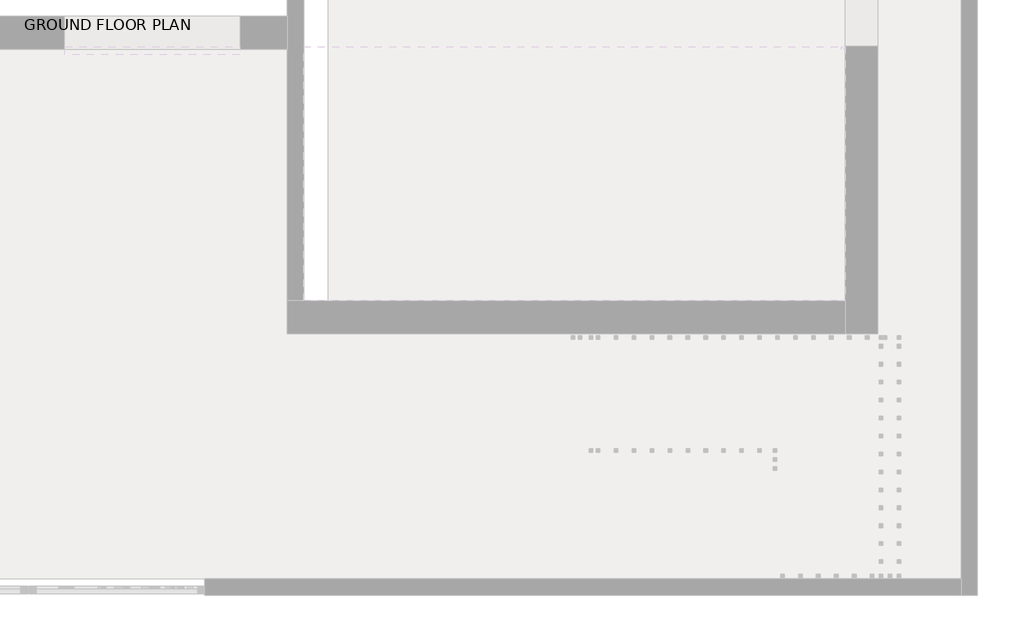
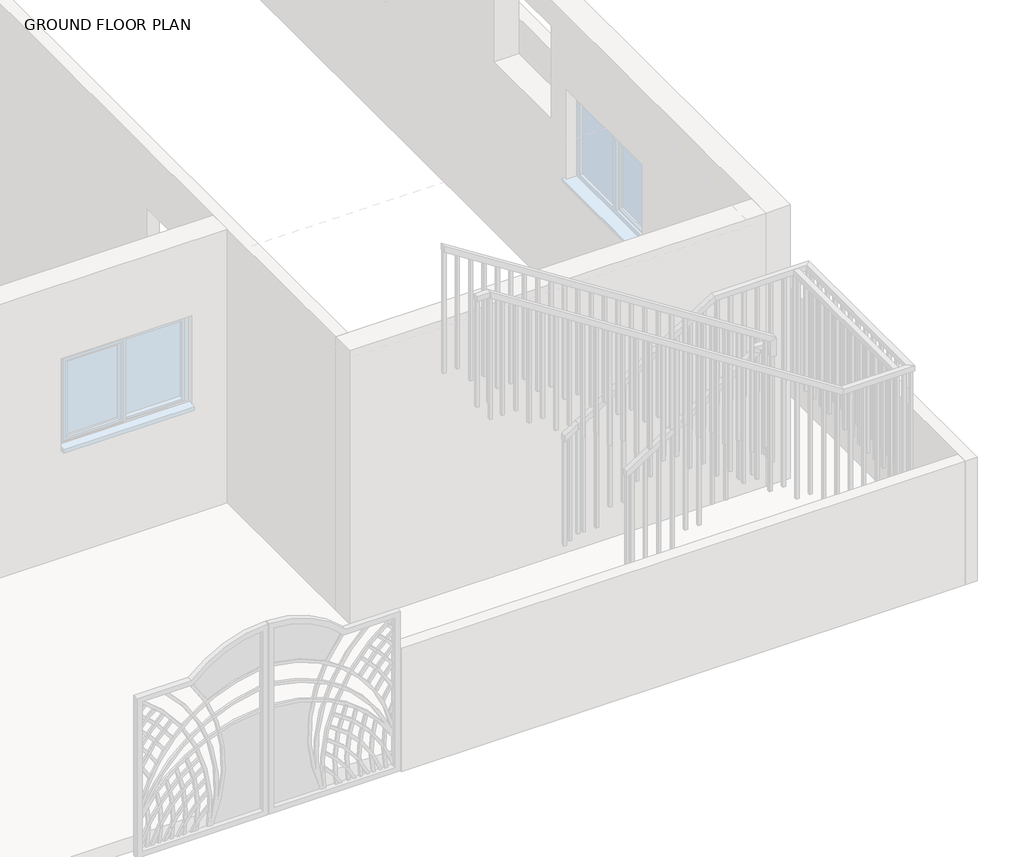
# One storey, part 15 of 23: 2 railings.
"""IFC4 building model written with IfcOpenShell, lengths in millimetres."""

from ifc_helpers import new_model, si_unit, frame, origin, place, context, project, spatial, polyline, outline, extrude, faceted_brep, element, save

model = new_model("IFC4")

# Units and contexts
model_context = context("Model", 3, world=origin())
ifc_project = project(units=[si_unit("LENGTHUNIT", "METRE", prefix="MILLI")], contexts=[model_context])

# Site, building, storey
site = spatial("IfcSite", under=ifc_project)
building = spatial("IfcBuilding", under=site)
storey = spatial("IfcBuildingStorey", under=building, Name="GROUND FLOOR PLAN", Elevation=487.68)

# Railings
placement = place(None, origin())
element("IfcRailing", 1, ObjectType="1100mm", at=placement, inside=storey, context=model_context, shape_type="SolidModel", body=[
    faceted_brep([(-8680.149573, -11007.9255223, 1912.8), (-8680.149573, -11007.9255223, 1853.4423995), (-8680.149573, -11057.9255223, 1853.4423995), (-8680.149573, -11057.9255223, 1912.8), (-7484.3306254, -11007.9255223, 2677.8717446), (-7434.3306254, -11007.9255223, 2650.5035914), (-7434.3306254, -11057.9255223, 2650.5035914), (-7484.3306254, -11057.9255223, 2677.8717446), (-7484.3306254, -11007.9255223, 2725.6), (-7434.3306254, -11007.9255223, 2675.6), (-7434.3306254, -11057.9255223, 2675.6), (-7484.3306254, -11057.9255223, 2725.6), (-7359.3306254, -11007.9255223, 2725.6), (-7359.3306254, -11007.9255223, 2675.6), (-7409.3306254, -11057.9255223, 2675.6), (-7409.3306254, -11057.9255223, 2725.6), (-7359.3306254, -11132.9255223, 2725.6), (-7359.3306254, -11132.9255223, 2675.6), (-7409.3306254, -11132.9255223, 2675.6), (-7409.3306254, -11132.9255223, 2725.6), (-7359.3306254, -11134.9255223, 2725.6), (-7409.3306254, -11134.9255223, 2725.6), (-7409.3306254, -11184.9255223, 2675.6), (-7359.3306254, -11184.9255223, 2675.6)], [[[0, 1, 2, 3]], [[1, 0, 4, 5]], [[2, 1, 5, 6]], [[3, 2, 6, 7]], [[0, 3, 7, 4]], [[5, 4, 8, 9]], [[6, 5, 9, 10]], [[7, 6, 10, 11]], [[4, 7, 11, 8]], [[9, 8, 12, 13]], [[10, 9, 13, 14]], [[11, 10, 14, 15]], [[8, 11, 15, 12]], [[13, 12, 16, 17]], [[14, 13, 17, 18]], [[15, 14, 18, 19]], [[12, 15, 19, 16]], [[20, 21, 22, 23]], [[17, 16, 20, 23]], [[18, 17, 23, 22]], [[19, 18, 22, 21]], [[16, 19, 21, 20]]]),
    faceted_brep([(-7359.3306254, -11134.9255223, 2725.6), (-7359.3306254, -11184.9255223, 2675.6), (-7409.3306254, -11184.9255223, 2675.6), (-7409.3306254, -11134.9255223, 2725.6), (-7359.3306254, -11134.9255223, 2855.9055527), (-7409.3306254, -11134.9255223, 2828.5415543), (-7409.3306254, -11184.9255223, 2828.5415543), (-7359.3306254, -11184.9255223, 2855.9055527)], [[[0, 1, 2, 3]], [[4, 5, 6, 7]], [[1, 0, 4, 7]], [[2, 1, 7, 6]], [[3, 2, 6, 5]], [[0, 3, 5, 4]]]),
    faceted_brep([(-7359.3306254, -11184.9255223, 2855.9055527), (-7409.3306254, -11184.9255223, 2828.5415543), (-7409.3306254, -11134.9255223, 2828.5415543), (-7359.3306254, -11134.9255223, 2855.9055527), (-10457.8773536, -11184.9255223, 4838.88), (-10457.8773536, -11134.9255223, 4838.88), (-10457.8773536, -11134.9255223, 4779.517542), (-10457.8773536, -11184.9255223, 4779.517542)], [[[0, 1, 2, 3]], [[4, 5, 6, 7]], [[1, 0, 4, 7]], [[2, 1, 7, 6]], [[3, 2, 6, 5]], [[0, 3, 5, 4]]]),
    extrude(outline(polyline([(3576.32, -10434.3306254), (4764.4483614, -10434.3306254), (4780.4475912, -10459.3306254), (3576.32, -10459.3306254), (3576.32, -10434.3306254)])), frame((0.0, -11172.4255223, 0.0), z_axis=(0.0, 1.0, 0.0), x_axis=(0.0, 0.0, 1.0)), (0.0, 0.0, 1.0), 25.0),
    extrude(outline(polyline([(3576.32, -10309.3306254), (4684.4522123, -10309.3306254), (4700.4514422, -10334.3306254), (3576.32, -10334.3306254), (3576.32, -10309.3306254)])), frame((0.0, -11172.4255223, 0.0), z_axis=(0.0, 1.0, 0.0), x_axis=(0.0, 0.0, 1.0)), (0.0, 0.0, 1.0), 25.0),
    extrude(outline(polyline([(3413.76, -10184.3306254), (4604.4560633, -10184.3306254), (4620.4552931, -10209.3306254), (3413.76, -10209.3306254), (3413.76, -10184.3306254)])), frame((0.0, -11172.4255223, 0.0), z_axis=(0.0, 1.0, 0.0), x_axis=(0.0, 0.0, 1.0)), (0.0, 0.0, 1.0), 25.0),
    extrude(outline(polyline([(3413.76, -10059.3306254), (4524.4599142, -10059.3306254), (4540.459144, -10084.3306254), (3413.76, -10084.3306254), (3413.76, -10059.3306254)])), frame((0.0, -11172.4255223, 0.0), z_axis=(0.0, 1.0, 0.0), x_axis=(0.0, 0.0, 1.0)), (0.0, 0.0, 1.0), 25.0),
    extrude(outline(polyline([(3251.2, -9934.3306254), (4444.4637652, -9934.3306254), (4460.462995, -9959.3306254), (3251.2, -9959.3306254), (3251.2, -9934.3306254)])), frame((0.0, -11172.4255223, 0.0), z_axis=(0.0, 1.0, 0.0), x_axis=(0.0, 0.0, 1.0)), (0.0, 0.0, 1.0), 25.0),
    extrude(outline(polyline([(3251.2, -9809.3306254), (4364.4676161, -9809.3306254), (4380.4668459, -9834.3306254), (3251.2, -9834.3306254), (3251.2, -9809.3306254)])), frame((0.0, -11172.4255223, 0.0), z_axis=(0.0, 1.0, 0.0), x_axis=(0.0, 0.0, 1.0)), (0.0, 0.0, 1.0), 25.0),
    extrude(outline(polyline([(3251.2, -9684.3306254), (4284.4714671, -9684.3306254), (4300.4706969, -9709.3306254), (3251.2, -9709.3306254), (3251.2, -9684.3306254)])), frame((0.0, -11172.4255223, 0.0), z_axis=(0.0, 1.0, 0.0), x_axis=(0.0, 0.0, 1.0)), (0.0, 0.0, 1.0), 25.0),
    extrude(outline(polyline([(3088.64, -9559.3306254), (4204.475318, -9559.3306254), (4220.4745478, -9584.3306254), (3088.64, -9584.3306254), (3088.64, -9559.3306254)])), frame((0.0, -11172.4255223, 0.0), z_axis=(0.0, 1.0, 0.0), x_axis=(0.0, 0.0, 1.0)), (0.0, 0.0, 1.0), 25.0),
    extrude(outline(polyline([(3088.64, -9434.3306254), (4124.479169, -9434.3306254), (4140.4783988, -9459.3306254), (3088.64, -9459.3306254), (3088.64, -9434.3306254)])), frame((0.0, -11172.4255223, 0.0), z_axis=(0.0, 1.0, 0.0), x_axis=(0.0, 0.0, 1.0)), (0.0, 0.0, 1.0), 25.0),
    extrude(outline(polyline([(2926.08, -9309.3306254), (4044.4830199, -9309.3306254), (4060.4822497, -9334.3306254), (2926.08, -9334.3306254), (2926.08, -9309.3306254)])), frame((0.0, -11172.4255223, 0.0), z_axis=(0.0, 1.0, 0.0), x_axis=(0.0, 0.0, 1.0)), (0.0, 0.0, 1.0), 25.0),
    extrude(outline(polyline([(2926.08, -9184.3306254), (3964.4868709, -9184.3306254), (3980.4861007, -9209.3306254), (2926.08, -9209.3306254), (2926.08, -9184.3306254)])), frame((0.0, -11172.4255223, 0.0), z_axis=(0.0, 1.0, 0.0), x_axis=(0.0, 0.0, 1.0)), (0.0, 0.0, 1.0), 25.0),
    extrude(outline(polyline([(2763.52, -9059.3306254), (3884.4907218, -9059.3306254), (3900.4899516, -9084.3306254), (2763.52, -9084.3306254), (2763.52, -9059.3306254)])), frame((0.0, -11172.4255223, 0.0), z_axis=(0.0, 1.0, 0.0), x_axis=(0.0, 0.0, 1.0)), (0.0, 0.0, 1.0), 25.0),
    extrude(outline(polyline([(2763.52, -8934.3306254), (3804.4945728, -8934.3306254), (3820.4938026, -8959.3306254), (2763.52, -8959.3306254), (2763.52, -8934.3306254)])), frame((0.0, -11172.4255223, 0.0), z_axis=(0.0, 1.0, 0.0), x_axis=(0.0, 0.0, 1.0)), (0.0, 0.0, 1.0), 25.0),
    extrude(outline(polyline([(2600.96, -8809.3306254), (3724.4984237, -8809.3306254), (3740.4976535, -8834.3306254), (2600.96, -8834.3306254), (2600.96, -8809.3306254)])), frame((0.0, -11172.4255223, 0.0), z_axis=(0.0, 1.0, 0.0), x_axis=(0.0, 0.0, 1.0)), (0.0, 0.0, 1.0), 25.0),
    extrude(outline(polyline([(2600.96, -8684.3306254), (3644.5022747, -8684.3306254), (3660.5015045, -8709.3306254), (2600.96, -8709.3306254), (2600.96, -8684.3306254)])), frame((0.0, -11172.4255223, 0.0), z_axis=(0.0, 1.0, 0.0), x_axis=(0.0, 0.0, 1.0)), (0.0, 0.0, 1.0), 25.0),
    extrude(outline(polyline([(2438.4, -8559.3306254), (3564.5061256, -8559.3306254), (3580.5053554, -8584.3306254), (2438.4, -8584.3306254), (2438.4, -8559.3306254)])), frame((0.0, -11172.4255223, 0.0), z_axis=(0.0, 1.0, 0.0), x_axis=(0.0, 0.0, 1.0)), (0.0, 0.0, 1.0), 25.0),
    extrude(outline(polyline([(2438.4, -8434.3306254), (3484.5099766, -8434.3306254), (3500.5092064, -8459.3306254), (2438.4, -8459.3306254), (2438.4, -8434.3306254)])), frame((0.0, -11172.4255223, 0.0), z_axis=(0.0, 1.0, 0.0), x_axis=(0.0, 0.0, 1.0)), (0.0, 0.0, 1.0), 25.0),
    extrude(outline(polyline([(2275.84, -8309.3306254), (3404.5138275, -8309.3306254), (3420.5130573, -8334.3306254), (2275.84, -8334.3306254), (2275.84, -8309.3306254)])), frame((0.0, -11172.4255223, 0.0), z_axis=(0.0, 1.0, 0.0), x_axis=(0.0, 0.0, 1.0)), (0.0, 0.0, 1.0), 25.0),
    extrude(outline(polyline([(2275.84, -8184.3306254), (3324.5176785, -8184.3306254), (3340.5169083, -8209.3306254), (2275.84, -8209.3306254), (2275.84, -8184.3306254)])), frame((0.0, -11172.4255223, 0.0), z_axis=(0.0, 1.0, 0.0), x_axis=(0.0, 0.0, 1.0)), (0.0, 0.0, 1.0), 25.0),
    extrude(outline(polyline([(2113.28, -8059.3306254), (3244.5215294, -8059.3306254), (3260.5207592, -8084.3306254), (2113.28, -8084.3306254), (2113.28, -8059.3306254)])), frame((0.0, -11172.4255223, 0.0), z_axis=(0.0, 1.0, 0.0), x_axis=(0.0, 0.0, 1.0)), (0.0, 0.0, 1.0), 25.0),
    extrude(outline(polyline([(2113.28, -7934.3306254), (3164.5253804, -7934.3306254), (3180.5246102, -7959.3306254), (2113.28, -7959.3306254), (2113.28, -7934.3306254)])), frame((0.0, -11172.4255223, 0.0), z_axis=(0.0, 1.0, 0.0), x_axis=(0.0, 0.0, 1.0)), (0.0, 0.0, 1.0), 25.0),
    extrude(outline(polyline([(1950.72, -7809.3306254), (3084.5292313, -7809.3306254), (3100.5284611, -7834.3306254), (1950.72, -7834.3306254), (1950.72, -7809.3306254)])), frame((0.0, -11172.4255223, 0.0), z_axis=(0.0, 1.0, 0.0), x_axis=(0.0, 0.0, 1.0)), (0.0, 0.0, 1.0), 25.0),
    extrude(outline(polyline([(1950.72, -7684.3306254), (3004.5330823, -7684.3306254), (3020.5323121, -7709.3306254), (1950.72, -7709.3306254), (1950.72, -7684.3306254)])), frame((0.0, -11172.4255223, 0.0), z_axis=(0.0, 1.0, 0.0), x_axis=(0.0, 0.0, 1.0)), (0.0, 0.0, 1.0), 25.0),
    extrude(outline(polyline([(1788.16, -7559.3306254), (2924.5369332, -7559.3306254), (2940.536163, -7584.3306254), (1788.16, -7584.3306254), (1788.16, -7559.3306254)])), frame((0.0, -11172.4255223, 0.0), z_axis=(0.0, 1.0, 0.0), x_axis=(0.0, 0.0, 1.0)), (0.0, 0.0, 1.0), 25.0),
    extrude(outline(polyline([(1788.16, -7434.3306254), (2844.5407841, -7434.3306254), (2860.540014, -7459.3306254), (1788.16, -7459.3306254), (1788.16, -7434.3306254)])), frame((0.0, -11172.4255223, 0.0), z_axis=(0.0, 1.0, 0.0), x_axis=(0.0, 0.0, 1.0)), (0.0, 0.0, 1.0), 25.0),
    extrude(outline(polyline([(-7396.8306254, -11082.9255223), (-7371.8306254, -11082.9255223), (-7371.8306254, -11107.9255223), (-7396.8306254, -11107.9255223), (-7396.8306254, -11082.9255223)])), frame((0.0, 0.0, 1625.6), z_axis=(0.0, 0.0, 1.0), x_axis=(1.0, 0.0, 0.0)), (0.0, 0.0, 1.0), 1050.0),
    extrude(outline(polyline([(2605.1944115, -7505.149573), (1463.04, -7505.149573), (1463.04, -7480.149573), (2621.1891352, -7480.149573), (2605.1944115, -7505.149573)])), frame((0.0, -11045.4255223, 0.0), z_axis=(0.0, 1.0, 0.0), x_axis=(0.0, 0.0, 1.0)), (0.0, 0.0, 1.0), 25.0),
    extrude(outline(polyline([(2525.2207932, -7630.149573), (1463.04, -7630.149573), (1463.04, -7605.149573), (2541.2155169, -7605.149573), (2525.2207932, -7630.149573)])), frame((0.0, -11045.4255223, 0.0), z_axis=(0.0, 1.0, 0.0), x_axis=(0.0, 0.0, 1.0)), (0.0, 0.0, 1.0), 25.0),
    extrude(outline(polyline([(2445.2471749, -7755.149573), (1300.48, -7755.149573), (1300.48, -7730.149573), (2461.2418986, -7730.149573), (2445.2471749, -7755.149573)])), frame((0.0, -11045.4255223, 0.0), z_axis=(0.0, 1.0, 0.0), x_axis=(0.0, 0.0, 1.0)), (0.0, 0.0, 1.0), 25.0),
    extrude(outline(polyline([(2365.2735566, -7880.149573), (1300.48, -7880.149573), (1300.48, -7855.149573), (2381.2682803, -7855.149573), (2365.2735566, -7880.149573)])), frame((0.0, -11045.4255223, 0.0), z_axis=(0.0, 1.0, 0.0), x_axis=(0.0, 0.0, 1.0)), (0.0, 0.0, 1.0), 25.0),
    extrude(outline(polyline([(2285.2999383, -8005.149573), (1137.92, -8005.149573), (1137.92, -7980.149573), (2301.294662, -7980.149573), (2285.2999383, -8005.149573)])), frame((0.0, -11045.4255223, 0.0), z_axis=(0.0, 1.0, 0.0), x_axis=(0.0, 0.0, 1.0)), (0.0, 0.0, 1.0), 25.0),
    extrude(outline(polyline([(2205.32632, -8130.149573), (1137.92, -8130.149573), (1137.92, -8105.149573), (2221.3210437, -8105.149573), (2205.32632, -8130.149573)])), frame((0.0, -11045.4255223, 0.0), z_axis=(0.0, 1.0, 0.0), x_axis=(0.0, 0.0, 1.0)), (0.0, 0.0, 1.0), 25.0),
    extrude(outline(polyline([(2125.3527017, -8255.149573), (975.36, -8255.149573), (975.36, -8230.149573), (2141.3474254, -8230.149573), (2125.3527017, -8255.149573)])), frame((0.0, -11045.4255223, 0.0), z_axis=(0.0, 1.0, 0.0), x_axis=(0.0, 0.0, 1.0)), (0.0, 0.0, 1.0), 25.0),
    extrude(outline(polyline([(2045.3790834, -8380.149573), (975.36, -8380.149573), (975.36, -8355.149573), (2061.3738071, -8355.149573), (2045.3790834, -8380.149573)])), frame((0.0, -11045.4255223, 0.0), z_axis=(0.0, 1.0, 0.0), x_axis=(0.0, 0.0, 1.0)), (0.0, 0.0, 1.0), 25.0),
    extrude(outline(polyline([(1965.4054651, -8505.149573), (812.8, -8505.149573), (812.8, -8480.149573), (1981.4001888, -8480.149573), (1965.4054651, -8505.149573)])), frame((0.0, -11045.4255223, 0.0), z_axis=(0.0, 1.0, 0.0), x_axis=(0.0, 0.0, 1.0)), (0.0, 0.0, 1.0), 25.0),
    extrude(outline(polyline([(1885.4318468, -8630.149573), (812.8, -8630.149573), (812.8, -8605.149573), (1901.4265705, -8605.149573), (1885.4318468, -8630.149573)])), frame((0.0, -11045.4255223, 0.0), z_axis=(0.0, 1.0, 0.0), x_axis=(0.0, 0.0, 1.0)), (0.0, 0.0, 1.0), 25.0),
    extrude(outline(polyline([(-7396.8306254, -11147.4255223), (-7371.8306254, -11147.4255223), (-7371.8306254, -11172.4255223), (-7396.8306254, -11172.4255223), (-7396.8306254, -11147.4255223)])), frame((0.0, 0.0, 1625.6), z_axis=(0.0, 0.0, 1.0), x_axis=(1.0, 0.0, 0.0)), (0.0, 0.0, 1.0), 1050.0),
    extrude(outline(polyline([(-7396.8306254, -11045.4255223), (-7396.8306254, -11020.4255223), (-7371.8306254, -11020.4255223), (-7371.8306254, -11045.4255223), (-7396.8306254, -11045.4255223)])), frame((0.0, 0.0, 1625.6), z_axis=(0.0, 0.0, 1.0), x_axis=(1.0, 0.0, 0.0)), (0.0, 0.0, 1.0), 1050.0),
    extrude(outline(polyline([(3576.32, -10432.8773536), (4763.5183122, -10432.8773536), (4779.517542, -10457.8773536), (3576.32, -10457.8773536), (3576.32, -10432.8773536)])), frame((0.0, -11172.4255223, 0.0), z_axis=(0.0, 1.0, 0.0), x_axis=(0.0, 0.0, 1.0)), (0.0, 0.0, 1.0), 25.0),
    extrude(outline(polyline([(1853.4423995, -8680.149573), (812.8, -8680.149573), (812.8, -8655.149573), (1869.4371231, -8655.149573), (1853.4423995, -8680.149573)])), frame((0.0, -11045.4255223, 0.0), z_axis=(0.0, 1.0, 0.0), x_axis=(0.0, 0.0, 1.0)), (0.0, 0.0, 1.0), 25.0),
])
element("IfcRailing", 2, ObjectType="1100mm", at=placement, inside=storey, context=model_context, shape_type="SolidModel", body=[
    faceted_brep([(-8680.149573, -10220.0521308, 1912.8), (-8680.149573, -10220.0521308, 1853.4423995), (-8680.149573, -10270.0521308, 1853.4423995), (-8680.149573, -10270.0521308, 1912.8), (-7409.7306254, -10220.0521308, 2725.6), (-7395.1045513, -10220.0521308, 2675.6), (-7395.1045513, -10270.0521308, 2675.6), (-7409.7306254, -10270.0521308, 2725.6), (-6495.8132565, -10220.0521308, 2725.6), (-6495.8132565, -10220.0521308, 2675.6), (-6545.8132565, -10270.0521308, 2675.6), (-6545.8132565, -10270.0521308, 2725.6), (-6495.8132565, -11933.6860066, 2725.6), (-6495.8132565, -11933.6860066, 2675.6), (-6545.8132565, -11883.6860066, 2675.6), (-6545.8132565, -11883.6860066, 2725.6), (-7155.718398, -11933.6860066, 2725.6), (-7170.3479429, -11933.6860066, 2675.6), (-7170.3479429, -11883.6860066, 2675.6), (-7155.718398, -11883.6860066, 2725.6), (-10457.8773536, -11933.6860066, 4838.88), (-10457.8773536, -11883.6860066, 4838.88), (-10457.8773536, -11883.6860066, 4779.517542), (-10457.8773536, -11933.6860066, 4779.517542)], [[[0, 1, 2, 3]], [[1, 0, 4, 5]], [[2, 1, 5, 6]], [[3, 2, 6, 7]], [[0, 3, 7, 4]], [[5, 4, 8, 9]], [[6, 5, 9, 10]], [[7, 6, 10, 11]], [[4, 7, 11, 8]], [[9, 8, 12, 13]], [[10, 9, 13, 14]], [[11, 10, 14, 15]], [[8, 11, 15, 12]], [[13, 12, 16, 17]], [[14, 13, 17, 18]], [[15, 14, 18, 19]], [[12, 15, 19, 16]], [[20, 21, 22, 23]], [[17, 16, 20, 23]], [[18, 17, 23, 22]], [[19, 18, 22, 21]], [[16, 19, 21, 20]]]),
    extrude(outline(polyline([(4691.8007425, -10320.8132565), (4707.7999723, -10345.8132565), (3576.32, -10345.8132565), (3576.32, -10320.8132565), (4691.8007425, -10320.8132565)])), frame((0.0, -11921.1860066, 0.0), z_axis=(0.0, 1.0, 0.0), x_axis=(0.0, 0.0, 1.0)), (0.0, 0.0, 1.0), 25.0),
    extrude(outline(polyline([(4611.8045935, -10195.8132565), (4627.8038233, -10220.8132565), (3576.32, -10220.8132565), (3576.32, -10195.8132565), (4611.8045935, -10195.8132565)])), frame((0.0, -11921.1860066, 0.0), z_axis=(0.0, 1.0, 0.0), x_axis=(0.0, 0.0, 1.0)), (0.0, 0.0, 1.0), 25.0),
    extrude(outline(polyline([(4531.8084444, -10070.8132565), (4547.8076742, -10095.8132565), (3413.76, -10095.8132565), (3413.76, -10070.8132565), (4531.8084444, -10070.8132565)])), frame((0.0, -11921.1860066, 0.0), z_axis=(0.0, 1.0, 0.0), x_axis=(0.0, 0.0, 1.0)), (0.0, 0.0, 1.0), 25.0),
    extrude(outline(polyline([(4451.8122954, -9945.8132565), (4467.8115252, -9970.8132565), (3413.76, -9970.8132565), (3413.76, -9945.8132565), (4451.8122954, -9945.8132565)])), frame((0.0, -11921.1860066, 0.0), z_axis=(0.0, 1.0, 0.0), x_axis=(0.0, 0.0, 1.0)), (0.0, 0.0, 1.0), 25.0),
    extrude(outline(polyline([(4371.8161463, -9820.8132565), (4387.8153761, -9845.8132565), (3251.2, -9845.8132565), (3251.2, -9820.8132565), (4371.8161463, -9820.8132565)])), frame((0.0, -11921.1860066, 0.0), z_axis=(0.0, 1.0, 0.0), x_axis=(0.0, 0.0, 1.0)), (0.0, 0.0, 1.0), 25.0),
    extrude(outline(polyline([(4291.8423995, -9695.8132565), (4307.8371231, -9720.8132565), (3251.2, -9720.8132565), (3251.2, -9695.8132565), (4291.8423995, -9695.8132565)])), frame((0.0, -11921.1860066, 0.0), z_axis=(0.0, 1.0, 0.0), x_axis=(0.0, 0.0, 1.0)), (0.0, 0.0, 1.0), 25.0),
    extrude(outline(polyline([(4211.8238482, -9570.8132565), (4227.823078, -9595.8132565), (3088.64, -9595.8132565), (3088.64, -9570.8132565), (4211.8238482, -9570.8132565)])), frame((0.0, -11921.1860066, 0.0), z_axis=(0.0, 1.0, 0.0), x_axis=(0.0, 0.0, 1.0)), (0.0, 0.0, 1.0), 25.0),
    extrude(outline(polyline([(4131.8276992, -9445.8132565), (4147.826929, -9470.8132565), (3088.64, -9470.8132565), (3088.64, -9445.8132565), (4131.8276992, -9445.8132565)])), frame((0.0, -11921.1860066, 0.0), z_axis=(0.0, 1.0, 0.0), x_axis=(0.0, 0.0, 1.0)), (0.0, 0.0, 1.0), 25.0),
    extrude(outline(polyline([(4051.8315501, -9320.8132565), (4067.8307799, -9345.8132565), (2926.08, -9345.8132565), (2926.08, -9320.8132565), (4051.8315501, -9320.8132565)])), frame((0.0, -11921.1860066, 0.0), z_axis=(0.0, 1.0, 0.0), x_axis=(0.0, 0.0, 1.0)), (0.0, 0.0, 1.0), 25.0),
    extrude(outline(polyline([(3971.835401, -9195.8132565), (3987.8346309, -9220.8132565), (2926.08, -9220.8132565), (2926.08, -9195.8132565), (3971.835401, -9195.8132565)])), frame((0.0, -11921.1860066, 0.0), z_axis=(0.0, 1.0, 0.0), x_axis=(0.0, 0.0, 1.0)), (0.0, 0.0, 1.0), 25.0),
    extrude(outline(polyline([(3891.839252, -9070.8132565), (3907.8384818, -9095.8132565), (2763.52, -9095.8132565), (2763.52, -9070.8132565), (3891.839252, -9070.8132565)])), frame((0.0, -11921.1860066, 0.0), z_axis=(0.0, 1.0, 0.0), x_axis=(0.0, 0.0, 1.0)), (0.0, 0.0, 1.0), 25.0),
    extrude(outline(polyline([(3811.8431029, -8945.8132565), (3827.8423328, -8970.8132565), (2763.52, -8970.8132565), (2763.52, -8945.8132565), (3811.8431029, -8945.8132565)])), frame((0.0, -11921.1860066, 0.0), z_axis=(0.0, 1.0, 0.0), x_axis=(0.0, 0.0, 1.0)), (0.0, 0.0, 1.0), 25.0),
    extrude(outline(polyline([(3731.8469539, -8820.8132565), (3747.8461837, -8845.8132565), (2600.96, -8845.8132565), (2600.96, -8820.8132565), (3731.8469539, -8820.8132565)])), frame((0.0, -11921.1860066, 0.0), z_axis=(0.0, 1.0, 0.0), x_axis=(0.0, 0.0, 1.0)), (0.0, 0.0, 1.0), 25.0),
    extrude(outline(polyline([(3651.8508048, -8695.8132565), (3667.8500347, -8720.8132565), (2600.96, -8720.8132565), (2600.96, -8695.8132565), (3651.8508048, -8695.8132565)])), frame((0.0, -11921.1860066, 0.0), z_axis=(0.0, 1.0, 0.0), x_axis=(0.0, 0.0, 1.0)), (0.0, 0.0, 1.0), 25.0),
    extrude(outline(polyline([(3571.8546558, -8570.8132565), (3587.8538856, -8595.8132565), (2438.4, -8595.8132565), (2438.4, -8570.8132565), (3571.8546558, -8570.8132565)])), frame((0.0, -11921.1860066, 0.0), z_axis=(0.0, 1.0, 0.0), x_axis=(0.0, 0.0, 1.0)), (0.0, 0.0, 1.0), 25.0),
    extrude(outline(polyline([(3491.8585067, -8445.8132565), (3507.8577365, -8470.8132565), (2438.4, -8470.8132565), (2438.4, -8445.8132565), (3491.8585067, -8445.8132565)])), frame((0.0, -11921.1860066, 0.0), z_axis=(0.0, 1.0, 0.0), x_axis=(0.0, 0.0, 1.0)), (0.0, 0.0, 1.0), 25.0),
    extrude(outline(polyline([(3411.8623577, -8320.8132565), (3427.8615875, -8345.8132565), (2275.84, -8345.8132565), (2275.84, -8320.8132565), (3411.8623577, -8320.8132565)])), frame((0.0, -11921.1860066, 0.0), z_axis=(0.0, 1.0, 0.0), x_axis=(0.0, 0.0, 1.0)), (0.0, 0.0, 1.0), 25.0),
    extrude(outline(polyline([(3331.8662086, -8195.8132565), (3347.8654384, -8220.8132565), (2275.84, -8220.8132565), (2275.84, -8195.8132565), (3331.8662086, -8195.8132565)])), frame((0.0, -11921.1860066, 0.0), z_axis=(0.0, 1.0, 0.0), x_axis=(0.0, 0.0, 1.0)), (0.0, 0.0, 1.0), 25.0),
    extrude(outline(polyline([(3251.8700596, -8070.8132565), (3267.8692894, -8095.8132565), (2113.28, -8095.8132565), (2113.28, -8070.8132565), (3251.8700596, -8070.8132565)])), frame((0.0, -11921.1860066, 0.0), z_axis=(0.0, 1.0, 0.0), x_axis=(0.0, 0.0, 1.0)), (0.0, 0.0, 1.0), 25.0),
    extrude(outline(polyline([(3171.8739105, -7945.8132565), (3187.8731403, -7970.8132565), (2113.28, -7970.8132565), (2113.28, -7945.8132565), (3171.8739105, -7945.8132565)])), frame((0.0, -11921.1860066, 0.0), z_axis=(0.0, 1.0, 0.0), x_axis=(0.0, 0.0, 1.0)), (0.0, 0.0, 1.0), 25.0),
    extrude(outline(polyline([(3091.8777615, -7820.8132565), (3107.8769913, -7845.8132565), (1950.72, -7845.8132565), (1950.72, -7820.8132565), (3091.8777615, -7820.8132565)])), frame((0.0, -11921.1860066, 0.0), z_axis=(0.0, 1.0, 0.0), x_axis=(0.0, 0.0, 1.0)), (0.0, 0.0, 1.0), 25.0),
    extrude(outline(polyline([(3011.8816124, -7695.8132565), (3027.8808422, -7720.8132565), (1950.72, -7720.8132565), (1950.72, -7695.8132565), (3011.8816124, -7695.8132565)])), frame((0.0, -11921.1860066, 0.0), z_axis=(0.0, 1.0, 0.0), x_axis=(0.0, 0.0, 1.0)), (0.0, 0.0, 1.0), 25.0),
    extrude(outline(polyline([(2931.8854634, -7570.8132565), (2947.8846932, -7595.8132565), (1788.16, -7595.8132565), (1788.16, -7570.8132565), (2931.8854634, -7570.8132565)])), frame((0.0, -11921.1860066, 0.0), z_axis=(0.0, 1.0, 0.0), x_axis=(0.0, 0.0, 1.0)), (0.0, 0.0, 1.0), 25.0),
    extrude(outline(polyline([(2851.8893143, -7445.8132565), (2867.8885441, -7470.8132565), (1788.16, -7470.8132565), (1788.16, -7445.8132565), (2851.8893143, -7445.8132565)])), frame((0.0, -11921.1860066, 0.0), z_axis=(0.0, 1.0, 0.0), x_axis=(0.0, 0.0, 1.0)), (0.0, 0.0, 1.0), 25.0),
    extrude(outline(polyline([(2771.8931653, -7320.8132565), (2787.8923951, -7345.8132565), (1625.6, -7345.8132565), (1625.6, -7320.8132565), (2771.8931653, -7320.8132565)])), frame((0.0, -11921.1860066, 0.0), z_axis=(0.0, 1.0, 0.0), x_axis=(0.0, 0.0, 1.0)), (0.0, 0.0, 1.0), 25.0),
    extrude(outline(polyline([(2691.8970162, -7195.8132565), (2707.896246, -7220.8132565), (1625.6, -7220.8132565), (1625.6, -7195.8132565), (2691.8970162, -7195.8132565)])), frame((0.0, -11921.1860066, 0.0), z_axis=(0.0, 1.0, 0.0), x_axis=(0.0, 0.0, 1.0)), (0.0, 0.0, 1.0), 25.0),
    extrude(outline(polyline([(-7070.8132565, -11921.1860066), (-7095.8132565, -11921.1860066), (-7095.8132565, -11896.1860066), (-7070.8132565, -11896.1860066), (-7070.8132565, -11921.1860066)])), frame((0.0, 0.0, 1625.6), z_axis=(0.0, 0.0, 1.0), x_axis=(1.0, 0.0, 0.0)), (0.0, 0.0, 1.0), 1050.0),
    extrude(outline(polyline([(-6945.8132565, -11921.1860066), (-6970.8132565, -11921.1860066), (-6970.8132565, -11896.1860066), (-6945.8132565, -11896.1860066), (-6945.8132565, -11921.1860066)])), frame((0.0, 0.0, 1625.6), z_axis=(0.0, 0.0, 1.0), x_axis=(1.0, 0.0, 0.0)), (0.0, 0.0, 1.0), 1050.0),
    extrude(outline(polyline([(-6820.8132565, -11921.1860066), (-6845.8132565, -11921.1860066), (-6845.8132565, -11896.1860066), (-6820.8132565, -11896.1860066), (-6820.8132565, -11921.1860066)])), frame((0.0, 0.0, 1625.6), z_axis=(0.0, 0.0, 1.0), x_axis=(1.0, 0.0, 0.0)), (0.0, 0.0, 1.0), 1050.0),
    extrude(outline(polyline([(-6695.8132565, -11921.1860066), (-6720.8132565, -11921.1860066), (-6720.8132565, -11896.1860066), (-6695.8132565, -11896.1860066), (-6695.8132565, -11921.1860066)])), frame((0.0, 0.0, 1625.6), z_axis=(0.0, 0.0, 1.0), x_axis=(1.0, 0.0, 0.0)), (0.0, 0.0, 1.0), 1050.0),
    extrude(outline(polyline([(-6570.8132565, -11921.1860066), (-6595.8132565, -11921.1860066), (-6595.8132565, -11896.1860066), (-6570.8132565, -11896.1860066), (-6570.8132565, -11921.1860066)])), frame((0.0, 0.0, 1625.6), z_axis=(0.0, 0.0, 1.0), x_axis=(1.0, 0.0, 0.0)), (0.0, 0.0, 1.0), 1050.0),
    extrude(outline(polyline([(-6508.3132565, -11795.0521308), (-6508.3132565, -11820.0521308), (-6533.3132565, -11820.0521308), (-6533.3132565, -11795.0521308), (-6508.3132565, -11795.0521308)])), frame((0.0, 0.0, 1625.6), z_axis=(0.0, 0.0, 1.0), x_axis=(1.0, 0.0, 0.0)), (0.0, 0.0, 1.0), 1050.0),
    extrude(outline(polyline([(-6508.3132565, -11670.0521308), (-6508.3132565, -11695.0521308), (-6533.3132565, -11695.0521308), (-6533.3132565, -11670.0521308), (-6508.3132565, -11670.0521308)])), frame((0.0, 0.0, 1625.6), z_axis=(0.0, 0.0, 1.0), x_axis=(1.0, 0.0, 0.0)), (0.0, 0.0, 1.0), 1050.0),
    extrude(outline(polyline([(-6508.3132565, -11545.0521308), (-6508.3132565, -11570.0521308), (-6533.3132565, -11570.0521308), (-6533.3132565, -11545.0521308), (-6508.3132565, -11545.0521308)])), frame((0.0, 0.0, 1625.6), z_axis=(0.0, 0.0, 1.0), x_axis=(1.0, 0.0, 0.0)), (0.0, 0.0, 1.0), 1050.0),
    extrude(outline(polyline([(-6508.3132565, -11420.0521308), (-6508.3132565, -11445.0521308), (-6533.3132565, -11445.0521308), (-6533.3132565, -11420.0521308), (-6508.3132565, -11420.0521308)])), frame((0.0, 0.0, 1625.6), z_axis=(0.0, 0.0, 1.0), x_axis=(1.0, 0.0, 0.0)), (0.0, 0.0, 1.0), 1050.0),
    extrude(outline(polyline([(-6508.3132565, -11295.0521308), (-6508.3132565, -11320.0521308), (-6533.3132565, -11320.0521308), (-6533.3132565, -11295.0521308), (-6508.3132565, -11295.0521308)])), frame((0.0, 0.0, 1625.6), z_axis=(0.0, 0.0, 1.0), x_axis=(1.0, 0.0, 0.0)), (0.0, 0.0, 1.0), 1050.0),
    extrude(outline(polyline([(-6508.3132565, -11170.0521308), (-6508.3132565, -11195.0521308), (-6533.3132565, -11195.0521308), (-6533.3132565, -11170.0521308), (-6508.3132565, -11170.0521308)])), frame((0.0, 0.0, 1625.6), z_axis=(0.0, 0.0, 1.0), x_axis=(1.0, 0.0, 0.0)), (0.0, 0.0, 1.0), 1050.0),
    extrude(outline(polyline([(-6508.3132565, -11045.0521308), (-6508.3132565, -11070.0521308), (-6533.3132565, -11070.0521308), (-6533.3132565, -11045.0521308), (-6508.3132565, -11045.0521308)])), frame((0.0, 0.0, 1625.6), z_axis=(0.0, 0.0, 1.0), x_axis=(1.0, 0.0, 0.0)), (0.0, 0.0, 1.0), 1050.0),
    extrude(outline(polyline([(-6508.3132565, -10920.0521308), (-6508.3132565, -10945.0521308), (-6533.3132565, -10945.0521308), (-6533.3132565, -10920.0521308), (-6508.3132565, -10920.0521308)])), frame((0.0, 0.0, 1625.6), z_axis=(0.0, 0.0, 1.0), x_axis=(1.0, 0.0, 0.0)), (0.0, 0.0, 1.0), 1050.0),
    extrude(outline(polyline([(-6508.3132565, -10795.0521308), (-6508.3132565, -10820.0521308), (-6533.3132565, -10820.0521308), (-6533.3132565, -10795.0521308), (-6508.3132565, -10795.0521308)])), frame((0.0, 0.0, 1625.6), z_axis=(0.0, 0.0, 1.0), x_axis=(1.0, 0.0, 0.0)), (0.0, 0.0, 1.0), 1050.0),
    extrude(outline(polyline([(-6508.3132565, -10670.0521308), (-6508.3132565, -10695.0521308), (-6533.3132565, -10695.0521308), (-6533.3132565, -10670.0521308), (-6508.3132565, -10670.0521308)])), frame((0.0, 0.0, 1625.6), z_axis=(0.0, 0.0, 1.0), x_axis=(1.0, 0.0, 0.0)), (0.0, 0.0, 1.0), 1050.0),
    extrude(outline(polyline([(-6508.3132565, -10545.0521308), (-6508.3132565, -10570.0521308), (-6533.3132565, -10570.0521308), (-6533.3132565, -10545.0521308), (-6508.3132565, -10545.0521308)])), frame((0.0, 0.0, 1625.6), z_axis=(0.0, 0.0, 1.0), x_axis=(1.0, 0.0, 0.0)), (0.0, 0.0, 1.0), 1050.0),
    extrude(outline(polyline([(-6508.3132565, -10420.0521308), (-6508.3132565, -10445.0521308), (-6533.3132565, -10445.0521308), (-6533.3132565, -10420.0521308), (-6508.3132565, -10420.0521308)])), frame((0.0, 0.0, 1625.6), z_axis=(0.0, 0.0, 1.0), x_axis=(1.0, 0.0, 0.0)), (0.0, 0.0, 1.0), 1050.0),
    extrude(outline(polyline([(-6508.3132565, -10295.0521308), (-6508.3132565, -10320.0521308), (-6533.3132565, -10320.0521308), (-6533.3132565, -10295.0521308), (-6508.3132565, -10295.0521308)])), frame((0.0, 0.0, 1625.6), z_axis=(0.0, 0.0, 1.0), x_axis=(1.0, 0.0, 0.0)), (0.0, 0.0, 1.0), 1050.0),
    extrude(outline(polyline([(-6630.149573, -10232.5521308), (-6605.149573, -10232.5521308), (-6605.149573, -10257.5521308), (-6630.149573, -10257.5521308), (-6630.149573, -10232.5521308)])), frame((0.0, 0.0, 1625.6), z_axis=(0.0, 0.0, 1.0), x_axis=(1.0, 0.0, 0.0)), (0.0, 0.0, 1.0), 1050.0),
    extrude(outline(polyline([(-6755.149573, -10232.5521308), (-6730.149573, -10232.5521308), (-6730.149573, -10257.5521308), (-6755.149573, -10257.5521308), (-6755.149573, -10232.5521308)])), frame((0.0, 0.0, 1625.6), z_axis=(0.0, 0.0, 1.0), x_axis=(1.0, 0.0, 0.0)), (0.0, 0.0, 1.0), 1050.0),
    extrude(outline(polyline([(-6880.149573, -10232.5521308), (-6855.149573, -10232.5521308), (-6855.149573, -10257.5521308), (-6880.149573, -10257.5521308), (-6880.149573, -10232.5521308)])), frame((0.0, 0.0, 1625.6), z_axis=(0.0, 0.0, 1.0), x_axis=(1.0, 0.0, 0.0)), (0.0, 0.0, 1.0), 1050.0),
    extrude(outline(polyline([(-7005.149573, -10232.5521308), (-6980.149573, -10232.5521308), (-6980.149573, -10257.5521308), (-7005.149573, -10257.5521308), (-7005.149573, -10232.5521308)])), frame((0.0, 0.0, 1625.6), z_axis=(0.0, 0.0, 1.0), x_axis=(1.0, 0.0, 0.0)), (0.0, 0.0, 1.0), 1050.0),
    extrude(outline(polyline([(-7130.149573, -10232.5521308), (-7105.149573, -10232.5521308), (-7105.149573, -10257.5521308), (-7130.149573, -10257.5521308), (-7130.149573, -10232.5521308)])), frame((0.0, 0.0, 1625.6), z_axis=(0.0, 0.0, 1.0), x_axis=(1.0, 0.0, 0.0)), (0.0, 0.0, 1.0), 1050.0),
    extrude(outline(polyline([(-7255.149573, -10232.5521308), (-7230.149573, -10232.5521308), (-7230.149573, -10257.5521308), (-7255.149573, -10257.5521308), (-7255.149573, -10232.5521308)])), frame((0.0, 0.0, 1625.6), z_axis=(0.0, 0.0, 1.0), x_axis=(1.0, 0.0, 0.0)), (0.0, 0.0, 1.0), 1050.0),
    extrude(outline(polyline([(-7380.149573, -10232.5521308), (-7355.149573, -10232.5521308), (-7355.149573, -10257.5521308), (-7380.149573, -10257.5521308), (-7380.149573, -10232.5521308)])), frame((0.0, 0.0, 1625.6), z_axis=(0.0, 0.0, 1.0), x_axis=(1.0, 0.0, 0.0)), (0.0, 0.0, 1.0), 1050.0),
    extrude(outline(polyline([(1463.04, -7505.149573), (1463.04, -7480.149573), (2621.1891352, -7480.149573), (2605.1944115, -7505.149573), (1463.04, -7505.149573)])), frame((0.0, -10257.5521308, 0.0), z_axis=(0.0, 1.0, 0.0), x_axis=(0.0, 0.0, 1.0)), (0.0, 0.0, 1.0), 25.0),
    extrude(outline(polyline([(1463.04, -7630.149573), (1463.04, -7605.149573), (2541.2155169, -7605.149573), (2525.2207932, -7630.149573), (1463.04, -7630.149573)])), frame((0.0, -10257.5521308, 0.0), z_axis=(0.0, 1.0, 0.0), x_axis=(0.0, 0.0, 1.0)), (0.0, 0.0, 1.0), 25.0),
    extrude(outline(polyline([(1300.48, -7755.149573), (1300.48, -7730.149573), (2461.2418986, -7730.149573), (2445.2471749, -7755.149573), (1300.48, -7755.149573)])), frame((0.0, -10257.5521308, 0.0), z_axis=(0.0, 1.0, 0.0), x_axis=(0.0, 0.0, 1.0)), (0.0, 0.0, 1.0), 25.0),
    extrude(outline(polyline([(1300.48, -7880.149573), (1300.48, -7855.149573), (2381.2682803, -7855.149573), (2365.2735566, -7880.149573), (1300.48, -7880.149573)])), frame((0.0, -10257.5521308, 0.0), z_axis=(0.0, 1.0, 0.0), x_axis=(0.0, 0.0, 1.0)), (0.0, 0.0, 1.0), 25.0),
    extrude(outline(polyline([(1137.92, -8005.149573), (1137.92, -7980.149573), (2301.294662, -7980.149573), (2285.2999383, -8005.149573), (1137.92, -8005.149573)])), frame((0.0, -10257.5521308, 0.0), z_axis=(0.0, 1.0, 0.0), x_axis=(0.0, 0.0, 1.0)), (0.0, 0.0, 1.0), 25.0),
    extrude(outline(polyline([(1137.92, -8130.149573), (1137.92, -8105.149573), (2221.3210437, -8105.149573), (2205.32632, -8130.149573), (1137.92, -8130.149573)])), frame((0.0, -10257.5521308, 0.0), z_axis=(0.0, 1.0, 0.0), x_axis=(0.0, 0.0, 1.0)), (0.0, 0.0, 1.0), 25.0),
    extrude(outline(polyline([(975.36, -8255.149573), (975.36, -8230.149573), (2141.3474254, -8230.149573), (2125.3527017, -8255.149573), (975.36, -8255.149573)])), frame((0.0, -10257.5521308, 0.0), z_axis=(0.0, 1.0, 0.0), x_axis=(0.0, 0.0, 1.0)), (0.0, 0.0, 1.0), 25.0),
    extrude(outline(polyline([(975.36, -8380.149573), (975.36, -8355.149573), (2061.3738071, -8355.149573), (2045.3790834, -8380.149573), (975.36, -8380.149573)])), frame((0.0, -10257.5521308, 0.0), z_axis=(0.0, 1.0, 0.0), x_axis=(0.0, 0.0, 1.0)), (0.0, 0.0, 1.0), 25.0),
    extrude(outline(polyline([(812.8, -8505.149573), (812.8, -8480.149573), (1981.4001888, -8480.149573), (1965.4054651, -8505.149573), (812.8, -8505.149573)])), frame((0.0, -10257.5521308, 0.0), z_axis=(0.0, 1.0, 0.0), x_axis=(0.0, 0.0, 1.0)), (0.0, 0.0, 1.0), 25.0),
    extrude(outline(polyline([(812.8, -8630.149573), (812.8, -8605.149573), (1901.4265705, -8605.149573), (1885.4318468, -8630.149573), (812.8, -8630.149573)])), frame((0.0, -10257.5521308, 0.0), z_axis=(0.0, 1.0, 0.0), x_axis=(0.0, 0.0, 1.0)), (0.0, 0.0, 1.0), 25.0),
    extrude(outline(polyline([(-6508.3132565, -11896.1860066), (-6508.3132565, -11921.1860066), (-6533.3132565, -11921.1860066), (-6533.3132565, -11896.1860066), (-6508.3132565, -11896.1860066)])), frame((0.0, 0.0, 1625.6), z_axis=(0.0, 0.0, 1.0), x_axis=(1.0, 0.0, 0.0)), (0.0, 0.0, 1.0), 1050.0),
    extrude(outline(polyline([(-6533.3132565, -10232.5521308), (-6508.3132565, -10232.5521308), (-6508.3132565, -10257.5521308), (-6533.3132565, -10257.5521308), (-6533.3132565, -10232.5521308)])), frame((0.0, 0.0, 1625.6), z_axis=(0.0, 0.0, 1.0), x_axis=(1.0, 0.0, 0.0)), (0.0, 0.0, 1.0), 1050.0),
    extrude(outline(polyline([(4763.5183122, -10432.8773536), (4779.517542, -10457.8773536), (3576.32, -10457.8773536), (3576.32, -10432.8773536), (4763.5183122, -10432.8773536)])), frame((0.0, -11921.1860066, 0.0), z_axis=(0.0, 1.0, 0.0), x_axis=(0.0, 0.0, 1.0)), (0.0, 0.0, 1.0), 25.0),
    extrude(outline(polyline([(812.8, -8680.149573), (812.8, -8655.149573), (1869.4371231, -8655.149573), (1853.4423995, -8680.149573), (812.8, -8680.149573)])), frame((0.0, -10257.5521308, 0.0), z_axis=(0.0, 1.0, 0.0), x_axis=(0.0, 0.0, 1.0)), (0.0, 0.0, 1.0), 25.0),
])

save(model, "model.ifc")

# Revit data of these elements
# Type "1100mm"
#   built-in parameter 1008612 = 0.019685 (stored number, unit not read)
#   built-in parameter 1008611 = 0.019685 (stored number, unit not read)
#   built-in parameter 1008609 = 0.902231 (stored number, unit not read)
#   built-in parameter 1008604 = 0.19685 (stored number, unit not read)
#   built-in parameter 1008603 = 0.164042 (stored number, unit not read)
#   Railing Height = 3.608924 ft
#   built-in parameter 1008630 = 2
#   built-in parameter 1008610 = 2
#   built-in parameter 1008608 = 1
#   built-in parameter 1008618 = Baluster_Square : 25mm
# Elements 1, 2 (IfcRailing, "1100mm")
#   Phase Created = New Construction
